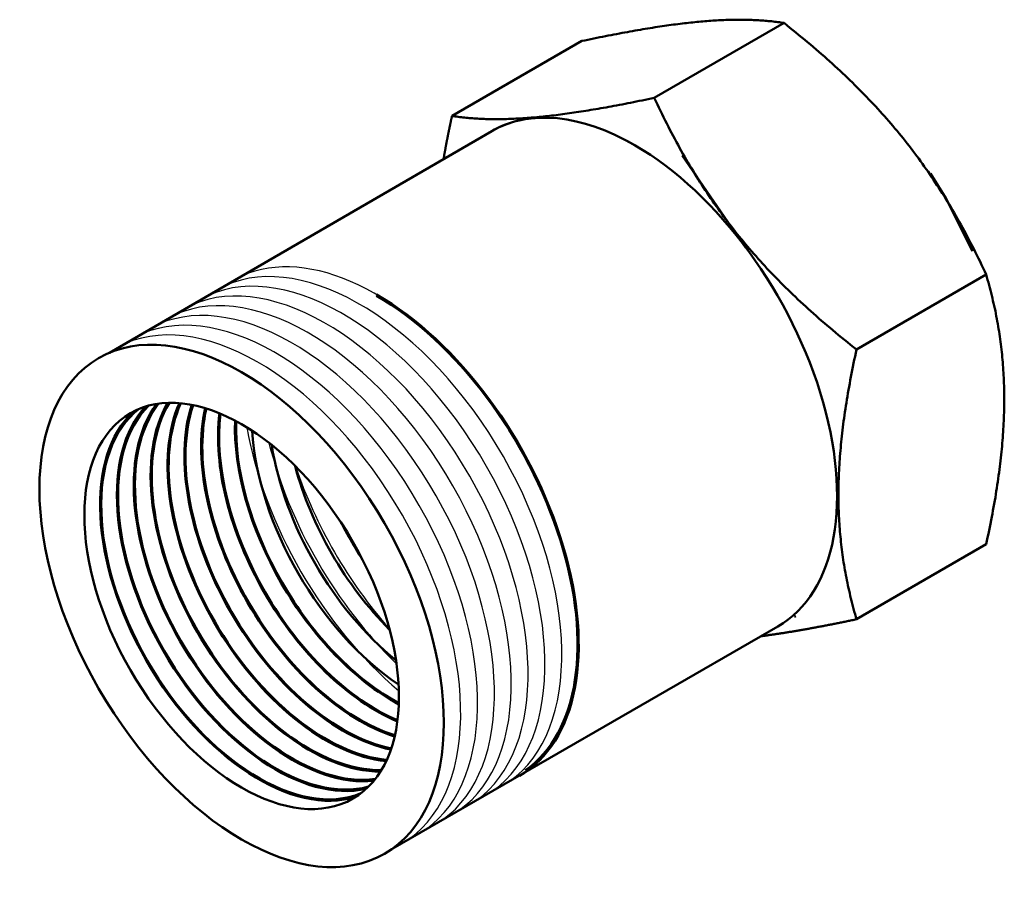
# Model space of a CAD drawing. Units: millimetres. Extents: x 0.2 to 76.1, y -3.5 to 64.3.
import ezdxf

# ---------------------------------------------------------------- set-up
doc = ezdxf.new("R2010")
doc.units = ezdxf.units.MM
doc.header["$MEASUREMENT"] = 0
doc.layers.add('M-OUTL', color=7, linetype='Continuous', lineweight=50)
doc.layers.add('M-THRD', color=2, linetype='Continuous', lineweight=25)

msp = doc.modelspace()

# ---------------------------------------------------------------- linework, layer by layer
at = {"layer": 'M-OUTL'}
for p, q in [((49.158, 58.251), (59.164, 64.028)), ((43.576, 62.636), (33.57, 56.859)), ((7.165, 38.61), (36.632, 55.69)), ((56.207, 46.732), (51.305, 53.8)), ((70.468, 52.427), (71.65, 50.52)), ((73.697, 46.438), (71.65, 50.52)), ((71.65, 50.52), (71.65, 50.52)), ((74.753, 44.636), (64.747, 38.859)), ((64.747, 18.074), (74.753, 23.851)), ((29.008, 0.421), (58.682, 17.509)), ((58.689, 17.513), (58.779, 17.566))]:
    msp.add_line(p, q, dxfattribs=at)
for points in [[(59.164, 64.028), (59.044, 64.044), (58.924, 64.06), (58.803, 64.076), (58.683, 64.092), (58.563, 64.108), (58.443, 64.124), (58.322, 64.14), (58.199, 64.151), (58.075, 64.162), (57.952, 64.174), (57.829, 64.185), (57.706, 64.196), (57.582, 64.208), (57.458, 64.218), (57.331, 64.225), (57.204, 64.231), (57.077, 64.238), (56.949, 64.245), (56.822, 64.252), (56.695, 64.258), (56.566, 64.263), (56.434, 64.266), (56.303, 64.268), (56.171, 64.27), (56.039, 64.272), (55.907, 64.274), (55.776, 64.277), (55.641, 64.276), (55.504, 64.274), (55.366, 64.272), (55.229, 64.269), (55.092, 64.267), (54.955, 64.265), (54.818, 64.262), (54.676, 64.257), (54.533, 64.25), (54.389, 64.243), (54.246, 64.236), (54.102, 64.229), (53.959, 64.222), (53.815, 64.215), (53.666, 64.205), (53.515, 64.193), (53.365, 64.182), (53.214, 64.17), (53.063, 64.159), (52.913, 64.147), (52.762, 64.136), (52.603, 64.12), (52.445, 64.103), (52.286, 64.087), (52.127, 64.071), (51.969, 64.055), (51.81, 64.039), (51.65, 64.022), (51.482, 64.001), (51.315, 63.98), (51.147, 63.959), (50.979, 63.938), (50.811, 63.917), (50.643, 63.896), (50.473, 63.874), (50.295, 63.848), (50.117, 63.822), (49.939, 63.797), (49.761, 63.771), (49.584, 63.745), (49.406, 63.719), (49.223, 63.691), (49.034, 63.66), (48.845, 63.629), (48.656, 63.599), (48.467, 63.568), (48.278, 63.537), (48.089, 63.506), (47.893, 63.472), (47.691, 63.436), (47.49, 63.4), (47.288, 63.364), (47.087, 63.328), (46.886, 63.292), (46.684, 63.255), (46.473, 63.215), (46.258, 63.174), (46.043, 63.132), (45.828, 63.091), (45.613, 63.049), (45.398, 63.007), (45.183, 62.966), (44.955, 62.919), (44.725, 62.872), (44.495, 62.825), (44.265, 62.777), (44.036, 62.73), (43.806, 62.683), (43.576, 62.636)], [(74.753, 44.636), (74.632, 44.885), (74.512, 45.134), (74.392, 45.384), (74.272, 45.633), (74.151, 45.883), (74.031, 46.132), (73.911, 46.38), (73.787, 46.617), (73.664, 46.854), (73.541, 47.091), (73.417, 47.328), (73.294, 47.565), (73.171, 47.801), (73.046, 48.035), (72.919, 48.261), (72.792, 48.487), (72.665, 48.713), (72.538, 48.938), (72.411, 49.164), (72.284, 49.39), (72.155, 49.612), (72.023, 49.828), (71.891, 50.044), (71.759, 50.26), (71.628, 50.476), (71.496, 50.692), (71.364, 50.908), (71.229, 51.119), (71.092, 51.327), (70.955, 51.535), (70.818, 51.742), (70.681, 51.95), (70.543, 52.158), (70.406, 52.366), (70.265, 52.568), (70.121, 52.769), (69.978, 52.969), (69.834, 53.17), (69.691, 53.371), (69.547, 53.571), (69.404, 53.772), (69.254, 53.967), (69.104, 54.162), (68.953, 54.357), (68.803, 54.551), (68.652, 54.746), (68.501, 54.941), (68.351, 55.136), (68.192, 55.326), (68.033, 55.516), (67.875, 55.706), (67.716, 55.896), (67.557, 56.086), (67.399, 56.276), (67.239, 56.466), (67.071, 56.652), (66.903, 56.839), (66.735, 57.025), (66.567, 57.212), (66.4, 57.398), (66.232, 57.585), (66.061, 57.771), (65.883, 57.955), (65.706, 58.139), (65.528, 58.323), (65.35, 58.508), (65.172, 58.692), (64.994, 58.876), (64.812, 59.06), (64.622, 59.243), (64.433, 59.426), (64.244, 59.609), (64.055, 59.792), (63.866, 59.975), (63.677, 60.158), (63.481, 60.341), (63.28, 60.524), (63.078, 60.706), (62.877, 60.889), (62.675, 61.072), (62.474, 61.255), (62.273, 61.438), (62.061, 61.622), (61.846, 61.806), (61.631, 61.99), (61.416, 62.174), (61.201, 62.358), (60.986, 62.542), (60.771, 62.725), (60.544, 62.911), (60.314, 63.097), (60.084, 63.284), (59.854, 63.47), (59.624, 63.656), (59.394, 63.842), (59.164, 64.028)], [(33.57, 56.859), (33.69, 56.843), (33.81, 56.827), (33.931, 56.811), (34.051, 56.795), (34.171, 56.779), (34.291, 56.762), (34.412, 56.747), (34.535, 56.736), (34.658, 56.724), (34.782, 56.713), (34.905, 56.702), (35.028, 56.69), (35.152, 56.679), (35.276, 56.669), (35.403, 56.662), (35.53, 56.655), (35.657, 56.649), (35.784, 56.642), (35.912, 56.635), (36.039, 56.628), (36.168, 56.623), (36.3, 56.621), (36.431, 56.619), (36.563, 56.617), (36.695, 56.615), (36.827, 56.612), (36.958, 56.61), (37.093, 56.611), (37.23, 56.613), (37.367, 56.615), (37.505, 56.618), (37.642, 56.62), (37.779, 56.622), (37.916, 56.625), (38.058, 56.63), (38.201, 56.637), (38.345, 56.644), (38.488, 56.651), (38.632, 56.658), (38.775, 56.665), (38.919, 56.671), (39.068, 56.682), (39.219, 56.694), (39.369, 56.705), (39.52, 56.717), (39.671, 56.728), (39.821, 56.74), (39.972, 56.751), (40.13, 56.767), (40.289, 56.783), (40.448, 56.8), (40.607, 56.816), (40.765, 56.832), (40.924, 56.848), (41.084, 56.865), (41.252, 56.886), (41.419, 56.907), (41.587, 56.928), (41.755, 56.949), (41.923, 56.969), (42.09, 56.99), (42.261, 57.013), (42.439, 57.039), (42.617, 57.064), (42.795, 57.09), (42.973, 57.116), (43.15, 57.142), (43.328, 57.168), (43.511, 57.196), (43.7, 57.226), (43.889, 57.257), (44.078, 57.288), (44.267, 57.319), (44.456, 57.35), (44.645, 57.381), (44.841, 57.415), (45.043, 57.451), (45.244, 57.487), (45.446, 57.523), (45.647, 57.559), (45.848, 57.595), (46.05, 57.631), (46.261, 57.671), (46.476, 57.713), (46.691, 57.755), (46.906, 57.796), (47.121, 57.838), (47.336, 57.879), (47.551, 57.921), (47.779, 57.967), (48.009, 58.015), (48.239, 58.062), (48.469, 58.109), (48.699, 58.157), (48.929, 58.204), (49.158, 58.251)], [(49.158, 58.251), (49.279, 58.002), (49.399, 57.752), (49.519, 57.503), (49.639, 57.253), (49.76, 57.004), (49.88, 56.755), (50, 56.507), (50.124, 56.27), (50.247, 56.033), (50.37, 55.796), (50.494, 55.559), (50.617, 55.322), (50.74, 55.085), (50.865, 54.852), (50.992, 54.626), (51.119, 54.4), (51.246, 54.174), (51.373, 53.948), (51.5, 53.723), (51.627, 53.497), (51.756, 53.275), (51.888, 53.059), (52.02, 52.843), (52.152, 52.627), (52.283, 52.411), (52.415, 52.195), (52.547, 51.979), (52.682, 51.767), (52.819, 51.56), (52.956, 51.352), (53.093, 51.144), (53.23, 50.937), (53.368, 50.729), (53.505, 50.521), (53.646, 50.319), (53.79, 50.118), (53.933, 49.917), (54.077, 49.717), (54.22, 49.516), (54.364, 49.316), (54.507, 49.115), (54.657, 48.919), (54.807, 48.725), (54.958, 48.53), (55.108, 48.335), (55.259, 48.141), (55.41, 47.946), (55.56, 47.751), (55.719, 47.561), (55.878, 47.371), (56.036, 47.181), (56.195, 46.991), (56.354, 46.801), (56.512, 46.611), (56.672, 46.421), (56.84, 46.235), (57.008, 46.048), (57.176, 45.862), (57.343, 45.675), (57.511, 45.488), (57.679, 45.302), (57.85, 45.116), (58.027, 44.932), (58.205, 44.748), (58.383, 44.563), (58.561, 44.379), (58.739, 44.195), (58.917, 44.011), (59.099, 43.827), (59.288, 43.644), (59.477, 43.461), (59.667, 43.278), (59.856, 43.095), (60.045, 42.912), (60.234, 42.729), (60.43, 42.546), (60.631, 42.363), (60.833, 42.18), (61.034, 41.997), (61.235, 41.814), (61.437, 41.632), (61.638, 41.449), (61.849, 41.265), (62.064, 41.081), (62.279, 40.897), (62.494, 40.713), (62.709, 40.529), (62.924, 40.345), (63.139, 40.161), (63.367, 39.975), (63.597, 39.789), (63.827, 39.603), (64.057, 39.417), (64.287, 39.231), (64.517, 39.045), (64.747, 38.859)], [(33.57, 56.859), (33.562, 56.823), (33.554, 56.787), (33.546, 56.75), (33.539, 56.714), (33.531, 56.678), (33.523, 56.642), (33.515, 56.606), (33.507, 56.57), (33.5, 56.535), (33.492, 56.499), (33.484, 56.463), (33.477, 56.427), (33.469, 56.391), (33.462, 56.356), (33.454, 56.32), (33.447, 56.285), (33.439, 56.249), (33.432, 56.213), (33.424, 56.178), (33.417, 56.142), (33.409, 56.107), (33.402, 56.072), (33.394, 56.036), (33.387, 56.001), (33.38, 55.966), (33.372, 55.93), (33.365, 55.895), (33.358, 55.86), (33.351, 55.825), (33.344, 55.79), (33.336, 55.755), (33.329, 55.72), (33.322, 55.685), (33.315, 55.649), (33.308, 55.615), (33.301, 55.58), (33.294, 55.545), (33.287, 55.51), (33.28, 55.475), (33.273, 55.44), (33.266, 55.406), (33.259, 55.371), (33.252, 55.336), (33.245, 55.302), (33.238, 55.267), (33.231, 55.233), (33.225, 55.198), (33.218, 55.163), (33.211, 55.129), (33.204, 55.095), (33.198, 55.06), (33.191, 55.026), (33.184, 54.992), (33.178, 54.957), (33.171, 54.923), (33.164, 54.889), (33.158, 54.855), (33.151, 54.821), (33.145, 54.787), (33.138, 54.752), (33.132, 54.718), (33.125, 54.684), (33.119, 54.65), (33.112, 54.616), (33.106, 54.583), (33.1, 54.549), (33.093, 54.515), (33.087, 54.481), (33.081, 54.447), (33.074, 54.413), (33.068, 54.38), (33.062, 54.346), (33.056, 54.312), (33.05, 54.279), (33.043, 54.245), (33.037, 54.211), (33.031, 54.178), (33.025, 54.145), (33.019, 54.111), (33.013, 54.078), (33.007, 54.044), (33.001, 54.011), (32.995, 53.977), (32.989, 53.944), (32.983, 53.911), (32.977, 53.878), (32.971, 53.844), (32.965, 53.811), (32.959, 53.778), (32.954, 53.745), (32.948, 53.712), (32.942, 53.679), (32.936, 53.646), (32.931, 53.613), (32.925, 53.58), (32.919, 53.547)], [(74.753, 23.851), (74.807, 24.116), (74.862, 24.382), (74.917, 24.647), (74.972, 24.912), (75.027, 25.177), (75.082, 25.442), (75.135, 25.705), (75.181, 25.957), (75.227, 26.209), (75.273, 26.461), (75.319, 26.713), (75.365, 26.965), (75.41, 27.217), (75.454, 27.466), (75.491, 27.706), (75.528, 27.947), (75.565, 28.187), (75.602, 28.428), (75.639, 28.668), (75.677, 28.909), (75.71, 29.145), (75.739, 29.375), (75.767, 29.606), (75.796, 29.836), (75.825, 30.066), (75.853, 30.297), (75.882, 30.527), (75.906, 30.753), (75.926, 30.974), (75.947, 31.196), (75.967, 31.418), (75.987, 31.64), (76.008, 31.861), (76.028, 32.083), (76.042, 32.3), (76.055, 32.514), (76.067, 32.729), (76.079, 32.943), (76.091, 33.158), (76.103, 33.372), (76.115, 33.587), (76.121, 33.796), (76.125, 34.005), (76.129, 34.213), (76.133, 34.422), (76.137, 34.63), (76.141, 34.839), (76.145, 35.047), (76.141, 35.251), (76.137, 35.455), (76.133, 35.659), (76.129, 35.863), (76.125, 36.067), (76.121, 36.27), (76.115, 36.474), (76.103, 36.674), (76.091, 36.875), (76.079, 37.075), (76.067, 37.276), (76.055, 37.476), (76.042, 37.677), (76.028, 37.876), (76.008, 38.075), (75.987, 38.273), (75.967, 38.471), (75.947, 38.669), (75.926, 38.868), (75.906, 39.066), (75.882, 39.264), (75.853, 39.461), (75.825, 39.658), (75.796, 39.856), (75.767, 40.053), (75.739, 40.25), (75.71, 40.448), (75.677, 40.645), (75.639, 40.843), (75.602, 41.04), (75.565, 41.238), (75.528, 41.436), (75.491, 41.633), (75.454, 41.831), (75.41, 42.029), (75.365, 42.228), (75.319, 42.427), (75.273, 42.626), (75.227, 42.826), (75.181, 43.025), (75.135, 43.224), (75.082, 43.425), (75.027, 43.627), (74.972, 43.828), (74.917, 44.03), (74.862, 44.232), (74.807, 44.434), (74.753, 44.636)], [(64.747, 38.859), (64.692, 38.594), (64.637, 38.328), (64.582, 38.063), (64.527, 37.798), (64.473, 37.533), (64.418, 37.268), (64.364, 37.005), (64.318, 36.753), (64.272, 36.501), (64.227, 36.249), (64.181, 35.997), (64.135, 35.745), (64.089, 35.493), (64.046, 35.244), (64.008, 35.004), (63.971, 34.763), (63.934, 34.523), (63.897, 34.282), (63.86, 34.042), (63.823, 33.801), (63.789, 33.565), (63.761, 33.335), (63.732, 33.104), (63.703, 32.874), (63.675, 32.644), (63.646, 32.413), (63.617, 32.183), (63.593, 31.957), (63.573, 31.736), (63.553, 31.514), (63.532, 31.292), (63.512, 31.07), (63.492, 30.849), (63.471, 30.627), (63.457, 30.41), (63.445, 30.196), (63.433, 29.981), (63.42, 29.767), (63.408, 29.552), (63.396, 29.338), (63.384, 29.123), (63.379, 28.914), (63.375, 28.705), (63.371, 28.497), (63.367, 28.288), (63.363, 28.08), (63.359, 27.871), (63.354, 27.663), (63.359, 27.459), (63.363, 27.255), (63.367, 27.051), (63.371, 26.847), (63.375, 26.643), (63.379, 26.44), (63.384, 26.236), (63.396, 26.036), (63.408, 25.835), (63.42, 25.635), (63.433, 25.434), (63.445, 25.234), (63.457, 25.033), (63.471, 24.834), (63.492, 24.635), (63.512, 24.437), (63.532, 24.239), (63.553, 24.041), (63.573, 23.842), (63.593, 23.644), (63.617, 23.446), (63.646, 23.249), (63.675, 23.052), (63.703, 22.854), (63.732, 22.657), (63.761, 22.46), (63.789, 22.262), (63.823, 22.065), (63.86, 21.867), (63.897, 21.67), (63.934, 21.472), (63.971, 21.274), (64.008, 21.077), (64.046, 20.879), (64.089, 20.681), (64.135, 20.482), (64.181, 20.283), (64.227, 20.084), (64.272, 19.884), (64.318, 19.685), (64.364, 19.486), (64.418, 19.285), (64.473, 19.083), (64.527, 18.882), (64.582, 18.68), (64.637, 18.478), (64.692, 18.276), (64.747, 18.074)], [(64.747, 18.074), (64.657, 18.056), (64.568, 18.037), (64.479, 18.018), (64.389, 18), (64.3, 17.981), (64.211, 17.962), (64.122, 17.944), (64.035, 17.926), (63.948, 17.908), (63.861, 17.89), (63.774, 17.872), (63.687, 17.855), (63.599, 17.837), (63.513, 17.819), (63.428, 17.802), (63.343, 17.785), (63.259, 17.768), (63.174, 17.751), (63.089, 17.734), (63.004, 17.717), (62.92, 17.7), (62.837, 17.684), (62.755, 17.668), (62.672, 17.652), (62.589, 17.636), (62.507, 17.62), (62.424, 17.603), (62.342, 17.588), (62.262, 17.572), (62.181, 17.557), (62.1, 17.542), (62.02, 17.526), (61.939, 17.511), (61.858, 17.495), (61.779, 17.481), (61.7, 17.466), (61.622, 17.451), (61.543, 17.437), (61.464, 17.422), (61.386, 17.408), (61.307, 17.393), (61.23, 17.379), (61.153, 17.365), (61.077, 17.352), (61, 17.338), (60.923, 17.324), (60.846, 17.31), (60.77, 17.296), (60.695, 17.283), (60.62, 17.27), (60.545, 17.257), (60.47, 17.244), (60.395, 17.231), (60.32, 17.218), (60.246, 17.205), (60.172, 17.193), (60.099, 17.181), (60.026, 17.169), (59.953, 17.156), (59.88, 17.144), (59.807, 17.132), (59.734, 17.12), (59.663, 17.108), (59.591, 17.097), (59.52, 17.085), (59.449, 17.074), (59.377, 17.062), (59.306, 17.051), (59.235, 17.039), (59.165, 17.029), (59.096, 17.018), (59.026, 17.007), (58.956, 16.996), (58.886, 16.986), (58.817, 16.975), (58.748, 16.964), (58.679, 16.954), (58.611, 16.944), (58.543, 16.934), (58.475, 16.924), (58.407, 16.914), (58.339, 16.904), (58.272, 16.894), (58.205, 16.885), (58.138, 16.876), (58.072, 16.866), (58.005, 16.857), (57.938, 16.848), (57.872, 16.838), (57.806, 16.83), (57.741, 16.821), (57.676, 16.812), (57.611, 16.804), (57.546, 16.795), (57.481, 16.787), (57.415, 16.778)]]:
    msp.add_lwpolyline(points, dxfattribs=at)
for centre, major_axis, start_param, end_param in [((47.666, 36.605), (11.023, -19.092), 2.356194, 3.141593), ((47.666, 36.605), (11.023, -19.092), 9.127346, 9.425772), ((47.666, 36.605), (11.023, -19.092), 6.282539, 8.676449), ((27.747, 25.105), (11.023, -19.092), 0, 2.356194), ((27.747, 25.105), (10.961, -18.986), 0.047158, 2.356194), ((18.654, 19.855), (8.573, -14.849), 3.217427, 6.207351), ((19.953, 20.605), (8.634, -14.955), 3.316417, 6.108361), ((19.953, 20.605), (8.573, -14.849), 3.293701, 6.131077), ((21.252, 21.355), (8.634, -14.955), 3.385329, 6.039449), ((21.252, 21.355), (8.573, -14.849), 3.370881, 6.053897), ((22.551, 22.105), (8.634, -14.955), 3.459564, 5.965214), ((22.551, 22.105), (8.573, -14.849), 3.44948, 5.975298), ((23.85, 22.855), (8.634, -14.955), 3.537359, 5.887419), ((23.85, 22.855), (8.573, -14.849), 3.5301, 5.894678), ((25.149, 23.605), (8.634, -14.955), 3.618657, 5.806121), ((25.149, 23.605), (8.573, -14.849), 3.613481, 5.811297), ((26.448, 24.355), (8.634, -14.955), 3.704065, 5.720713), ((26.448, 24.355), (8.573, -14.849), 3.700583, 5.724195), ((18.654, 19.855), (8.634, -14.955), 3.264096, 6.160682), ((27.747, 25.105), (8.634, -14.955), 3.794709, 5.630069), ((27.747, 25.105), (8.573, -14.849), 3.79273, 5.632048), ((29.046, 25.855), (8.634, -14.955), 3.89241, 5.532368), ((29.046, 25.855), (8.573, -14.849), 3.891885, 5.532893), ((30.346, 26.605), (8.634, -14.955), 4.000208, 5.42457), ((31.645, 27.355), (8.634, -14.955), 4.123819, 5.300959), ((32.944, 28.105), (8.634, -14.955), 4.276758, 5.14802), ((48.965, 37.355), (11.023, -19.092), 6.282539, 6.291403), ((19.953, 20.605), (11.023, -19.092), 6.224226, 6.225546)]:
    msp.add_ellipse(centre, major_axis=major_axis, ratio=0.57735, start_param=start_param, end_param=end_param, dxfattribs=at)
for major_axis in [(11.023, -19.092), (8.573, -14.849)]:
    msp.add_ellipse((17.355, 19.105), major_axis=major_axis, ratio=0.57735, dxfattribs=at)
at = {"layer": 'M-THRD'}
for centre, start_param, end_param in [((26.448, 24.355), 6.332407, 9.363893), ((27.747, 25.105), 8.092802, 9.365818), ((25.149, 23.605), 6.333911, 9.362027), ((23.85, 22.855), 6.335372, 9.360213), ((22.551, 22.105), 6.336795, 9.358448), ((21.252, 21.355), 6.33818, 9.356728), ((19.953, 20.605), 6.339533, 9.35505), ((18.654, 19.855), 6.340853, 9.353411), ((32.944, 28.105), 4.151499, 5.273279), ((34.243, 28.855), 4.249942, 5.174836), ((35.542, 29.605), 4.378209, 5.046569), ((36.841, 30.355), 4.618801, 4.805977)]:
    msp.add_ellipse(centre, major_axis=(11.023, -19.092), ratio=0.57735, start_param=start_param, end_param=end_param, dxfattribs=at)

doc.saveas('drawing.dxf')
